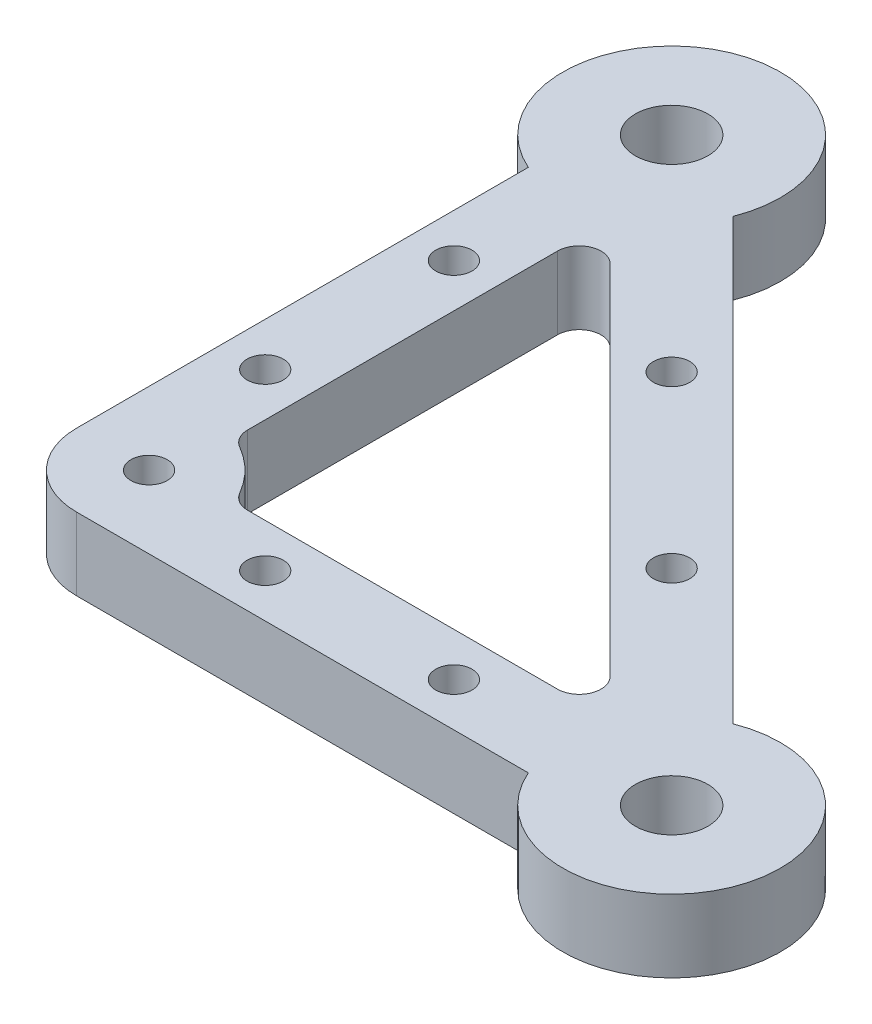
from build123d import *

# Parameters (mm, degrees)
WEB_PLATE_PROFILE_R          = 5
WEB_PLATE_PROFILE_R_2        = 2.5
WEB_PLATE_EXTRUDE_10MM_DEPTH = 5


with BuildPart() as part:
    # Web Plate Profile → Web Plate Extrude 10mm (new, symmetric)
    with BuildSketch(Plane(origin=(0, 0, 0), x_dir=(1, 0, 0), z_dir=(0, 1, 0))):
        with BuildLine():
            Line((-6, 4), (-6, 66.252272915))
            ThreePointArc((-6, 66.252272915), (-5.740251485, 93.858192988), (13.963751735, 74.52152964))
            Line((13.963751735, 74.52152964), (74.52152964, 13.963751735))
            ThreePointArc((74.52152964, 13.963751735), (93.858192988, -5.740251485), (66.252272915, -6))
            Line((66.252272915, -6), (4, -6))
            ThreePointArc((4, -6), (-3.071067812, -3.071067812), (-6, 4))
        make_face()
        with Locations(Location((0, 80, 0), (0, 0, 270))):
            Circle(WEB_PLATE_PROFILE_R, mode=Mode.SUBTRACT)
        with Locations(Location((80, 0, 0), (0, 0, 270))):
            Circle(WEB_PLATE_PROFILE_R, mode=Mode.SUBTRACT)
        with Locations(Location((4, 4, 0), (0, 0, 270))):
            Circle(WEB_PLATE_PROFILE_R_2, mode=Mode.SUBTRACT)
        with Locations(Location((50, 0, 0), (0, 0, 270))):
            Circle(WEB_PLATE_PROFILE_R_2, mode=Mode.SUBTRACT)
        with Locations(Location((24, 0, 0), (0, 0, 270))):
            Circle(WEB_PLATE_PROFILE_R_2, mode=Mode.SUBTRACT)
        with Locations(Location((0, 24, 0), (0, 0, 270))):
            Circle(WEB_PLATE_PROFILE_R_2, mode=Mode.SUBTRACT)
        with Locations(Location((0, 50, 0), (0, 0, 270))):
            Circle(WEB_PLATE_PROFILE_R_2, mode=Mode.SUBTRACT)
        with Locations(Location((28.284271247, 51.715728753, 0), (0, 0, 270))):
            Circle(WEB_PLATE_PROFILE_R_2, mode=Mode.SUBTRACT)
        with Locations(Location((51.715728753, 28.284271247, 0), (0, 0, 270))):
            Circle(WEB_PLATE_PROFILE_R_2, mode=Mode.SUBTRACT)
        with BuildLine():
            Line((11.121320344, 60.393398282), (60.393398282, 11.121320344))
            ThreePointArc((60.393398282, 11.121320344), (61.043716536, 7.851949703), (58.272077939, 6))
            Line((58.272077939, 6), (15.588457268, 6))
            ThreePointArc((15.588457268, 6), (14.088457268, 6.401923789), (12.990381057, 7.5))
            ThreePointArc((12.990381057, 7.5), (10.606601718, 10.606601718), (7.5, 12.990381057))
            ThreePointArc((7.5, 12.990381057), (6.401923789, 14.088457268), (6, 15.588457268))
            Line((6, 15.588457268), (6, 58.272077939))
            ThreePointArc((6, 58.272077939), (7.851949703, 61.043716536), (11.121320344, 60.393398282))
        make_face(mode=Mode.SUBTRACT)
    extrude(amount=WEB_PLATE_EXTRUDE_10MM_DEPTH, both=True)


solid = part.part
